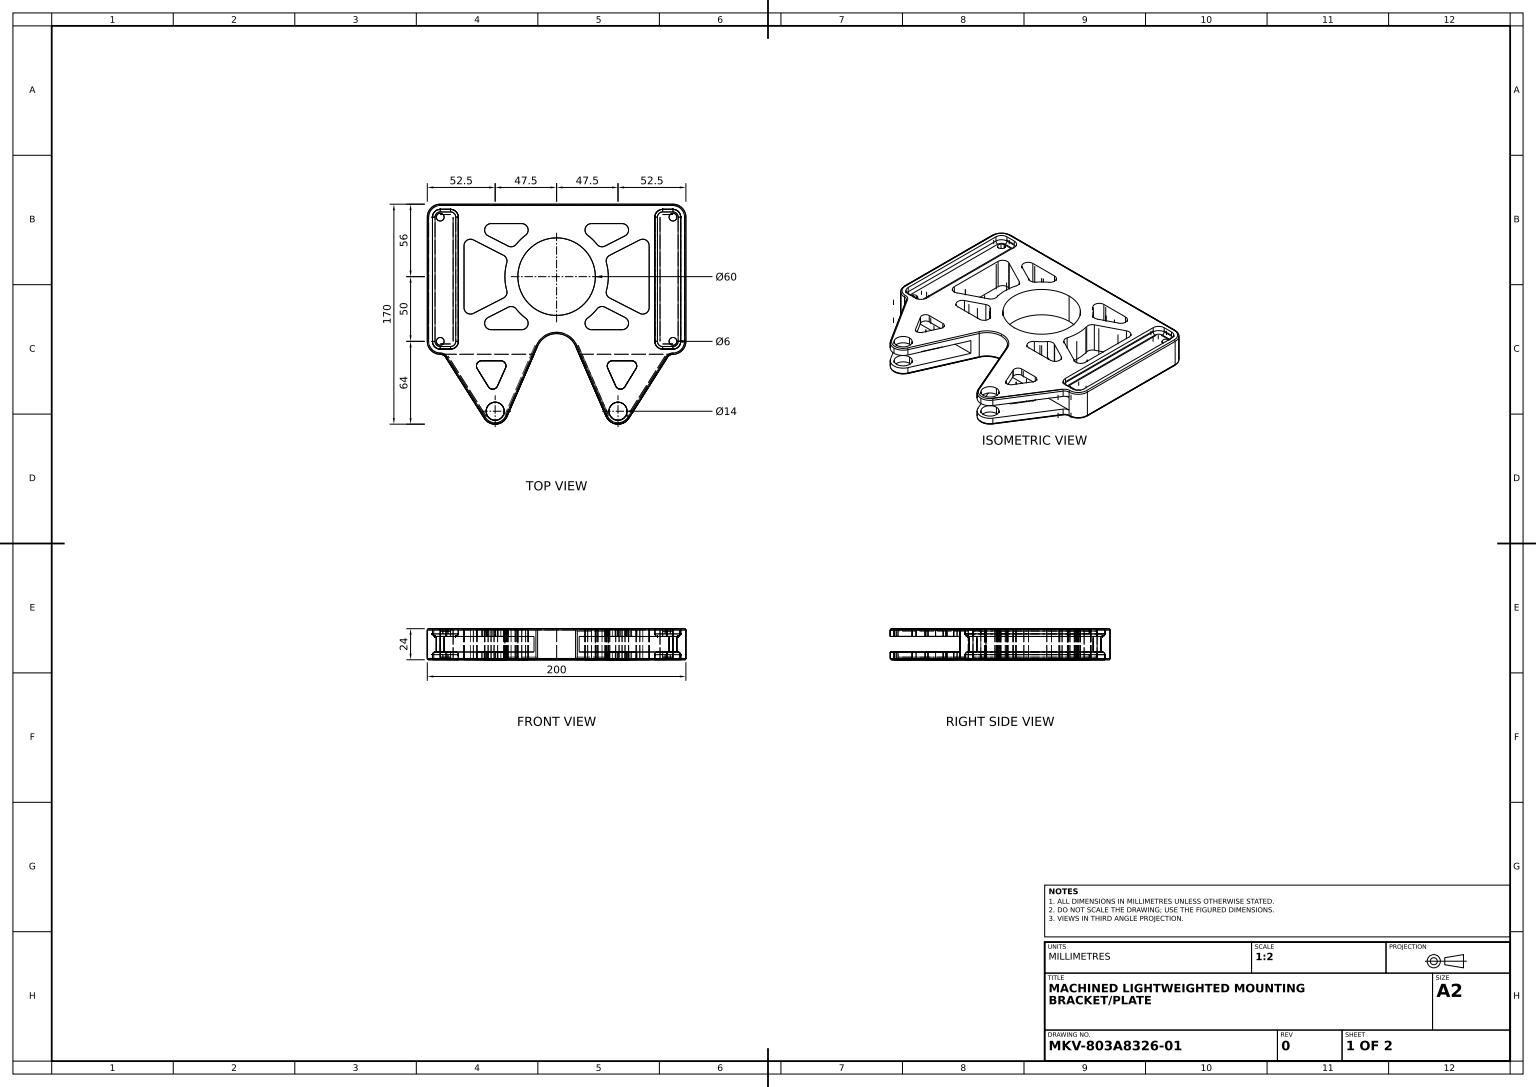
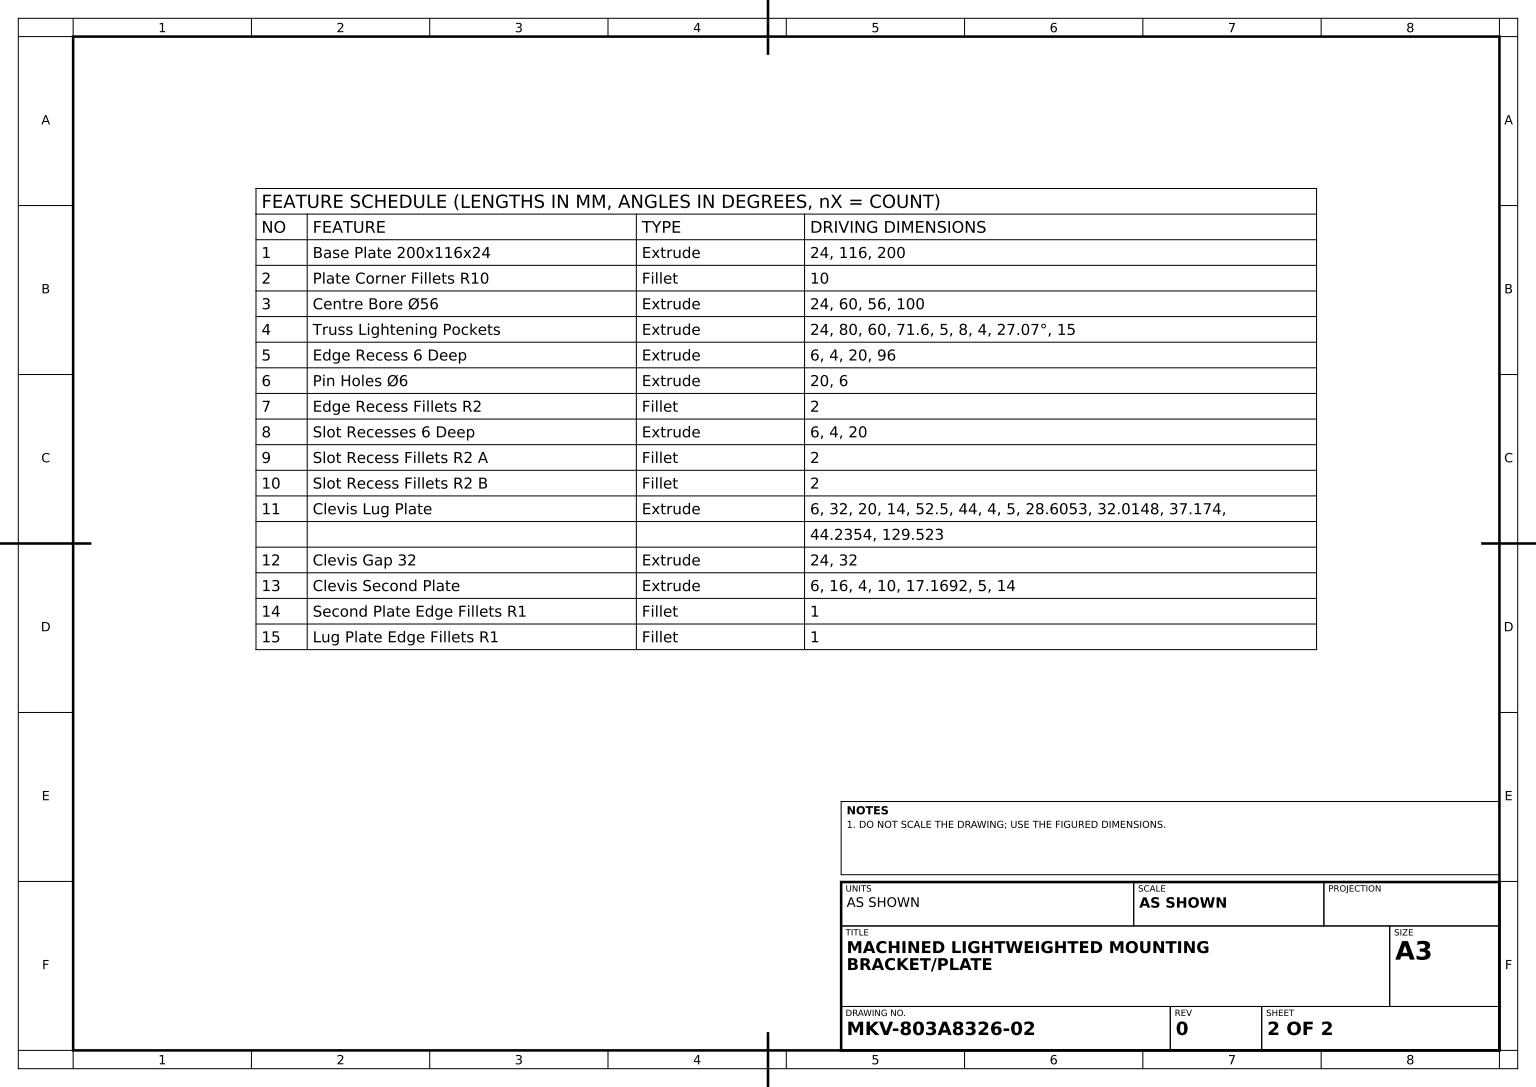
from build123d import *

# Parameters (mm, degrees)
BASE_PLATE_SKETCH_W            = 200
BASE_PLATE_SKETCH_H            = 116
BASE_PLATE_200X116X24_DEPTH    = 24
PLATE_CORNER_FILLETS_R10_R     = 10
CENTRE_BORE_SKETCH_R           = 30
CENTRE_BORE_56_DEPTH           = 24
TRUSS_LIGHTENING_POCKETS_DEPTH = 24
EDGE_RECESS_6_DEEP_DEPTH       = 6
PIN_HOLE_SKETCH_R              = 3
PIN_HOLES_6_DEPTH              = 20
EDGE_RECESS_FILLETS_R2_R       = 2
SLOT_START                     = -6
SLOT_RECESSES_6_DEEP_DEPTH     = 6
SLOT_RECESS_FILLETS_R2_A_R     = 2
SLOT_RECESS_FILLETS_R2_B_R     = 2
CLEVIS_LUG_PLATE_SKETCH_R      = 7
CLEVIS_LUG_PLATE_DEPTH         = 6
CLEVIS_GAP_32_DEPTH            = 24
CLEVIS_START                   = -6
CLEVIS_SECOND_PLATE_SKETCH_R   = 7
CLEVIS_SECOND_PLATE_DEPTH      = 6
SECOND_PLATE_EDGE_FILLETS_R1_R = 1
LUG_PLATE_EDGE_FILLETS_R1_R    = 1


with BuildPart() as part:
    # Base Plate Sketch → Base Plate 200x116x24 (new body)
    with BuildSketch(Plane(origin=(0, 0, 0), x_dir=(1, 0, 0), z_dir=(0, 1, 0))):
        Rectangle(BASE_PLATE_SKETCH_W, BASE_PLATE_SKETCH_H)
    extrude(amount=BASE_PLATE_200X116X24_DEPTH)

    # Plate Corner Fillets R10
    plate_corner_fillets_r10_edges = [part.edges().sort_by_distance(p)[0] for p in [
        (100, 12, 58),
        (-100, 12, 58),
        (-100, 12, -58),
        (100, 12, -58),
    ]]
    fillet(plate_corner_fillets_r10_edges, radius=PLATE_CORNER_FILLETS_R10_R)

    # Centre Bore Sketch → Centre Bore Ø56 (cut)
    with BuildSketch(Plane(origin=(0, 24, 0), x_dir=(1, 0, 0), z_dir=(0, 1, 0))):
        with Locations(Location((0, 2, 0), (0, 0, 270))):
            Circle(CENTRE_BORE_SKETCH_R)
    extrude(amount=-CENTRE_BORE_56_DEPTH, mode=Mode.SUBTRACT)

    # Truss Pocket Sketch → Truss Lightening Pockets (cut)
    with BuildSketch(Plane(origin=(0, 24, 0), x_dir=(1, 0, 0), z_dir=(0, 1, 0))):
        with BuildLine():
            ThreePointArc((-27, 43), (-22.25658351, 39.58113883), (-24, 34))
            ThreePointArc((-24, 34), (-27.851763511, 30.710264181), (-31.256881452, 26.960115422))
            ThreePointArc((-31.256881452, 26.960115422), (-34.110827486, 25.192303618), (-37.439546933, 25.627956439))
            Line((-37.439546933, 25.627956439), (-52.934945053, 33.547826589))
            ThreePointArc((-52.934945053, 33.547826589), (-55.520504186, 39.170284783), (-50.659389754, 43))
            Line((-50.659389754, 43), (-27, 43))
        make_face()
        with BuildLine():
            ThreePointArc((-41.080435411, 18.504478981), (-38.777551451, 16.061756728), (-38.538658409, 12.713160507))
            ThreePointArc((-38.538658409, 12.713160507), (-40, 2), (-38.538658409, -8.713160507))
            ThreePointArc((-38.538658409, -8.713160507), (-38.777551451, -12.061756728), (-41.080435411, -14.504478981))
            Line((-41.080435411, -14.504478981), (-64.324444701, -26.384750396))
            ThreePointArc((-64.324444701, -26.384750396), (-69.209810674, -26.19742027), (-71.6, -21.932576985))
            Line((-71.6, -21.932576985), (-71.6, 25.932576985))
            ThreePointArc((-71.6, 25.932576985), (-69.209810674, 30.19742027), (-64.324444701, 30.384750396))
            Line((-64.324444701, 30.384750396), (-41.080435411, 18.504478981))
        make_face()
        with BuildLine():
            ThreePointArc((31.256881452, 26.960115422), (27.851763511, 30.710264181), (24, 34))
            ThreePointArc((24, 34), (22.25658351, 39.58113883), (27, 43))
            Line((27, 43), (50.659389754, 43))
            ThreePointArc((50.659389754, 43), (55.520504186, 39.170284783), (52.934945053, 33.547826589))
            Line((52.934945053, 33.547826589), (37.439546933, 25.627956439))
            ThreePointArc((37.439546933, 25.627956439), (34.110827486, 25.192303618), (31.256881452, 26.960115422))
        make_face()
        with BuildLine():
            Line((40, 2), (71.6, 2))
            Line((71.6, 2), (71.6, 25.932576985))
            ThreePointArc((71.6, 25.932576985), (69.209810674, 30.19742027), (64.324444701, 30.384750396))
            Line((64.324444701, 30.384750396), (41.080435411, 18.504478981))
            ThreePointArc((41.080435411, 18.504478981), (38.777551451, 16.061756728), (38.538658409, 12.713160507))
            ThreePointArc((38.538658409, 12.713160507), (39.632980814, 7.40618459), (40, 2))
        make_face()
        with BuildLine():
            ThreePointArc((64.324444701, -26.384750396), (69.209810674, -26.19742027), (71.6, -21.932576985))
            Line((71.6, -21.932576985), (71.6, 2))
            Line((71.6, 2), (40, 2))
            ThreePointArc((40, 2), (39.632980814, -3.40618459), (38.538658409, -8.713160507))
            ThreePointArc((38.538658409, -8.713160507), (38.777551451, -12.061756728), (41.080435411, -14.504478981))
            Line((41.080435411, -14.504478981), (64.324444701, -26.384750396))
        make_face()
        with BuildLine():
            ThreePointArc((27, -39), (22.25658351, -35.58113883), (24, -30))
            ThreePointArc((24, -30), (27.851763511, -26.710264181), (31.256881452, -22.960115422))
            ThreePointArc((31.256881452, -22.960115422), (34.110827486, -21.192303618), (37.439546933, -21.627956439))
            Line((37.439546933, -21.627956439), (52.934945053, -29.547826589))
            ThreePointArc((52.934945053, -29.547826589), (55.520504186, -35.170284783), (50.659389754, -39))
            Line((50.659389754, -39), (27, -39))
        make_face()
        with BuildLine():
            ThreePointArc((-27, -39), (-22.25658351, -35.58113883), (-24, -30))
            ThreePointArc((-24, -30), (-27.851763511, -26.710264181), (-31.256881452, -22.960115422))
            ThreePointArc((-31.256881452, -22.960115422), (-34.110827486, -21.192303618), (-37.439546933, -21.627956439))
            Line((-37.439546933, -21.627956439), (-52.934945053, -29.547826589))
            ThreePointArc((-52.934945053, -29.547826589), (-55.520504186, -35.170284783), (-50.659389754, -39))
            Line((-50.659389754, -39), (-27, -39))
        make_face()
    extrude(amount=-TRUSS_LIGHTENING_POCKETS_DEPTH, mode=Mode.SUBTRACT)

    # Edge Recess Sketch → Edge Recess 6 Deep (cut)
    with BuildSketch(Plane(origin=(0, 24, 0), x_dir=(1, 0, 0), z_dir=(0, 1, 0))):
        with BuildLine():
            Line((82, -54), (90, -54))
            ThreePointArc((90, -54), (94.242640687, -52.242640687), (96, -48))
            Line((96, -48), (96, 48))
            ThreePointArc((96, 48), (94.242640687, 52.242640687), (90, 54))
            Line((90, 54), (82, 54))
            ThreePointArc((82, 54), (77.757359313, 52.242640687), (76, 48))
            Line((76, 48), (76, -48))
            ThreePointArc((76, -48), (77.757359313, -52.242640687), (82, -54))
        make_face()
        with BuildLine():
            Line((-76, 48), (-76, -48))
            ThreePointArc((-76, -48), (-77.757359313, -52.242640687), (-82, -54))
            Line((-82, -54), (-90, -54))
            ThreePointArc((-90, -54), (-94.242640687, -52.242640687), (-96, -48))
            Line((-96, -48), (-96, 48))
            ThreePointArc((-96, 48), (-94.242640687, 52.242640687), (-90, 54))
            Line((-90, 54), (-82, 54))
            ThreePointArc((-82, 54), (-77.757359313, 52.242640687), (-76, 48))
        make_face()
    extrude(amount=-EDGE_RECESS_6_DEEP_DEPTH, mode=Mode.SUBTRACT)

    # Pin Hole Sketch → Pin Holes Ø6 (cut)
    with BuildSketch(Plane(origin=(0, 18, 0), x_dir=(1, 0, 0), z_dir=(0, 1, 0))):
        with Locations(Location((90, 48, 0), (0, 0, 270))):
            Circle(PIN_HOLE_SKETCH_R)
        with Locations(Location((90, -48, 0), (0, 0, 270))):
            Circle(PIN_HOLE_SKETCH_R)
        with Locations(Location((-90, 48, 0), (0, 0, 270))):
            Circle(PIN_HOLE_SKETCH_R)
        with Locations(Location((-90, -48, 0), (0, 0, 270))):
            Circle(PIN_HOLE_SKETCH_R)
    extrude(amount=-PIN_HOLES_6_DEPTH, mode=Mode.SUBTRACT)

    # Edge Recess Fillets R2
    edge_recess_fillets_r2_edges = [part.edges().sort_by_distance(p)[0] for p in [
        (86, 18, 54),
        (77.757359313, 18, 52.242640687),
        (76, 18, 0),
        (86, 18, -54),
        (94.242640687, 18, 52.242640687),
        (77.757359313, 18, -52.242640687),
        (94.242640687, 18, -52.242640687),
        (96, 18, 0),
        (-96, 18, 0),
        (-94.242640687, 18, -52.242640687),
        (-77.757359313, 18, -52.242640687),
        (-76, 18, 0),
        (-77.757359313, 18, 52.242640687),
        (-86, 18, 54),
        (-94.242640687, 18, 52.242640687),
        (-86, 18, -54),
    ]]
    fillet(edge_recess_fillets_r2_edges, radius=EDGE_RECESS_FILLETS_R2_R)

    # Slot Recess Sketch → Slot Recesses 6 Deep (cut)
    with BuildSketch(Plane.XZ.offset(SLOT_START)):
        with BuildLine():
            Line((-96, -48), (-96, 48))
            ThreePointArc((-96, 48), (-94.242640687, 52.242640687), (-90, 54))
            Line((-90, 54), (-82, 54))
            ThreePointArc((-82, 54), (-77.757359313, 52.242640687), (-76, 48))
            Line((-76, 48), (-76, -48))
            ThreePointArc((-76, -48), (-77.757359313, -52.242640687), (-82, -54))
            Line((-82, -54), (-90, -54))
            ThreePointArc((-90, -54), (-94.242640687, -52.242640687), (-96, -48))
        make_face()
        with BuildLine():
            Line((90, -54), (82, -54))
            ThreePointArc((82, -54), (77.757359313, -52.242640687), (76, -48))
            Line((76, -48), (76, 48))
            ThreePointArc((76, 48), (77.757359313, 52.242640687), (82, 54))
            Line((82, 54), (90, 54))
            ThreePointArc((90, 54), (94.242640687, 52.242640687), (96, 48))
            Line((96, 48), (96, -48))
            ThreePointArc((96, -48), (94.242640687, -52.242640687), (90, -54))
        make_face()
    extrude(amount=SLOT_RECESSES_6_DEEP_DEPTH, mode=Mode.SUBTRACT)

    # Slot Recess Fillets R2 A
    slot_recess_fillets_r2_a_edges = [part.edges().sort_by_distance(p)[0] for p in [
        (-94.242640687, 6, 52.242640687),
        (-86, 6, 54),
        (-77.757359313, 6, 52.242640687),
        (-76, 6, 0),
        (-77.757359313, 6, -52.242640687),
        (-86, 6, -54),
        (-94.242640687, 6, -52.242640687),
        (-96, 6, 0),
    ]]
    fillet(slot_recess_fillets_r2_a_edges, radius=SLOT_RECESS_FILLETS_R2_A_R)

    # Slot Recess Fillets R2 B
    slot_recess_fillets_r2_b_edges = [part.edges().sort_by_distance(p)[0] for p in [
        (94.242640687, 6, 52.242640687),
        (96, 6, 0),
        (94.242640687, 6, -52.242640687),
        (86, 6, -54),
        (77.757359313, 6, -52.242640687),
        (76, 6, 0),
        (77.757359313, 6, 52.242640687),
        (86, 6, 54),
    ]]
    fillet(slot_recess_fillets_r2_b_edges, radius=SLOT_RECESS_FILLETS_R2_B_R)

    # Clevis Lug Plate Sketch → Clevis Lug Plate (add)
    # profile 1 of 2: a face of its own
    with BuildSketch(Plane(origin=(0, 0, 0), x_dir=(1, 0, 0), z_dir=(0, 1, 0))):
        with BuildLine():
            ThreePointArc((-90, -58), (-87.590708212, -58.618754391), (-85.777720374, -60.321874767))
            Line((-85.777720374, -60.321874767), (-55.944559251, -107.356250466))
            ThreePointArc((-55.944559251, -107.356250466), (-46.726594369, -111.970047328), (-38.330434827, -105.989871494))
            Line((-38.330434827, -105.989871494), (-17.44902806, -58))
            Line((-17.44902806, -58), (-90, -58))
        make_face()
        with Locations(Location((-47.5, -102, 0), (0, 0, 270))):
            Circle(CLEVIS_LUG_PLATE_SKETCH_R, mode=Mode.SUBTRACT)
        with BuildLine():
            Line((-52.82600088, -83.058899908), (-61.39472553, -69.091700081))
            ThreePointArc((-61.39472553, -69.091700081), (-61.475683559, -65.046388002), (-57.985210789, -63))
            Line((-57.985210789, -63), (-43.17473691, -63))
            ThreePointArc((-43.17473691, -63), (-39.818549541, -64.823763261), (-39.522807782, -68.631996828))
            Line((-39.522807782, -68.631996828), (-45.764557011, -82.599196656))
            ThreePointArc((-45.764557011, -82.599196656), (-49.156634346, -84.958750534), (-52.82600088, -83.058899908))
        make_face(mode=Mode.SUBTRACT)
    # profile 2 of 2: a face of its own
    with BuildSketch(Plane(origin=(0, 0, 0), x_dir=(1, 0, 0), z_dir=(0, 1, 0))):
        with BuildLine():
            Line((90, -58), (17.44902806, -58))
            Line((17.44902806, -58), (38.330434827, -105.989871494))
            ThreePointArc((38.330434827, -105.989871494), (46.726594369, -111.970047328), (55.944559251, -107.356250466))
            Line((55.944559251, -107.356250466), (85.777720374, -60.321874767))
            ThreePointArc((85.777720374, -60.321874767), (87.590708212, -58.618754391), (90, -58))
        make_face()
        with Locations(Location((47.5, -102, 0), (0, 0, 270))):
            Circle(CLEVIS_LUG_PLATE_SKETCH_R, mode=Mode.SUBTRACT)
        with BuildLine():
            ThreePointArc((52.82600088, -83.058899908), (49.156634346, -84.958750534), (45.764557011, -82.599196656))
            Line((45.764557011, -82.599196656), (39.522807782, -68.631996828))
            ThreePointArc((39.522807782, -68.631996828), (39.818549541, -64.823763261), (43.17473691, -63))
            Line((43.17473691, -63), (57.985210789, -63))
            ThreePointArc((57.985210789, -63), (61.475683559, -65.046388002), (61.39472553, -69.091700081))
            Line((61.39472553, -69.091700081), (52.82600088, -83.058899908))
        make_face(mode=Mode.SUBTRACT)
    extrude(amount=CLEVIS_LUG_PLATE_DEPTH)

    # Clevis Gap Sketch → Clevis Gap 32 (cut)
    with BuildSketch(Plane(origin=(0, 24, 0), x_dir=(1, 0, 0), z_dir=(0, 1, 0))):
        with BuildLine():
            Line((-17.44902806, -58), (-14.671304277, -51.61620561))
            ThreePointArc((-14.671304277, -51.61620561), (0, -42), (14.671304277, -51.61620561))
            Line((14.671304277, -51.61620561), (17.44902806, -58))
            Line((17.44902806, -58), (-17.44902806, -58))
        make_face()
    extrude(amount=-CLEVIS_GAP_32_DEPTH, mode=Mode.SUBTRACT)

    # Clevis Second Plate Sketch → Clevis Second Plate (add)
    # profile 1 of 2: a face of its own
    with BuildSketch(Plane(origin=(0, 24, 0), x_dir=(1, 0, 0), z_dir=(0, 1, 0)).offset(CLEVIS_START)):
        with BuildLine():
            Line((-17.44902806, -58), (-90, -58))
            ThreePointArc((-90, -58), (-87.590708212, -58.618754391), (-85.777720374, -60.321874767))
            Line((-85.777720374, -60.321874767), (-55.944559251, -107.356250466))
            ThreePointArc((-55.944559251, -107.356250466), (-46.726594369, -111.970047328), (-38.330434827, -105.989871494))
            Line((-38.330434827, -105.989871494), (-17.44902806, -58))
        make_face()
        with Locations(Location((-47.5, -102, 0), (0, 0, 270))):
            Circle(CLEVIS_SECOND_PLATE_SKETCH_R, mode=Mode.SUBTRACT)
        with BuildLine():
            ThreePointArc((-61.39472553, -69.091700081), (-61.475683559, -65.046388002), (-57.985210789, -63))
            Line((-57.985210789, -63), (-43.17473691, -63))
            ThreePointArc((-43.17473691, -63), (-39.818549541, -64.823763261), (-39.522807782, -68.631996828))
            Line((-39.522807782, -68.631996828), (-45.764557011, -82.599196656))
            ThreePointArc((-45.764557011, -82.599196656), (-48.765392722, -84.913853773), (-52.350692715, -83.685734684))
            Line((-52.350692715, -83.685734684), (-61.39472553, -69.091700081))
        make_face(mode=Mode.SUBTRACT)
    # profile 2 of 2: a face of its own
    with BuildSketch(Plane(origin=(0, 24, 0), x_dir=(1, 0, 0), z_dir=(0, 1, 0)).offset(CLEVIS_START)):
        with BuildLine():
            Line((90, -58), (17.44902806, -58))
            Line((17.44902806, -58), (38.330434827, -105.989871494))
            ThreePointArc((38.330434827, -105.989871494), (46.726594369, -111.970047328), (55.944559251, -107.356250466))
            Line((55.944559251, -107.356250466), (85.777720374, -60.321874767))
            ThreePointArc((85.777720374, -60.321874767), (87.590708212, -58.618754391), (90, -58))
        make_face()
        with Locations(Location((47.5, -102, 0), (0, 0, 270))):
            Circle(CLEVIS_SECOND_PLATE_SKETCH_R, mode=Mode.SUBTRACT)
        with BuildLine():
            Line((61.39472553, -69.091700081), (52.82600088, -83.058899908))
            ThreePointArc((52.82600088, -83.058899908), (49.156634346, -84.958750534), (45.764557011, -82.599196656))
            Line((45.764557011, -82.599196656), (39.522807782, -68.631996828))
            ThreePointArc((39.522807782, -68.631996828), (39.818549541, -64.823763261), (43.17473691, -63))
            Line((43.17473691, -63), (57.985210789, -63))
            ThreePointArc((57.985210789, -63), (61.475683559, -65.046388002), (61.39472553, -69.091700081))
        make_face(mode=Mode.SUBTRACT)
    extrude(amount=CLEVIS_SECOND_PLATE_DEPTH)

    # Second Plate Edge Fillets R1
    second_plate_edge_fillets_r1_edges = [part.edges().sort_by_distance(p)[0] for p in [
        (-100, 24, 0),
        (0, 24, -58),
        (100, 24, 0),
        (-97.071067812, 24, 55.071067812),
        (97.071067812, 24, 55.071067812),
        (97.071067812, 24, -55.071067812),
        (-97.071067812, 24, -55.071067812),
        (26.500869552, 24, 78.803038552),
        (0, 24, 42),
        (-26.500869552, 24, 78.803038552),
        (-70.861139813, 24, 83.839062616),
        (-46.726594369, 24, 111.970047328),
        (-87.590708212, 24, 58.618754391),
        (87.590708212, 24, 58.618754391),
        (46.726594369, 24, 111.970047328),
        (70.861139813, 24, 83.839062616),
    ]]
    fillet(second_plate_edge_fillets_r1_edges, radius=SECOND_PLATE_EDGE_FILLETS_R1_R)

    # Lug Plate Edge Fillets R1
    lug_plate_edge_fillets_r1_edges = [part.edges().sort_by_distance(p)[0] for p in [
        (-100, 0, 0),
        (100, 0, 0),
        (0, 0, -58),
        (-97.071067812, 0, 55.071067812),
        (97.071067812, 0, 55.071067812),
        (97.071067812, 0, -55.071067812),
        (-97.071067812, 0, -55.071067812),
        (-87.590708212, 0, 58.618754391),
        (-70.861139813, 0, 83.839062616),
        (-46.726594369, 0, 111.970047328),
        (-26.500869552, 0, 78.803038552),
        (87.590708212, 0, 58.618754391),
        (70.861139813, 0, 83.839062616),
        (46.726594369, 0, 111.970047328),
        (26.500869552, 0, 78.803038552),
        (0, 0, 42),
    ]]
    fillet(lug_plate_edge_fillets_r1_edges, radius=LUG_PLATE_EDGE_FILLETS_R1_R)


solid = part.part
